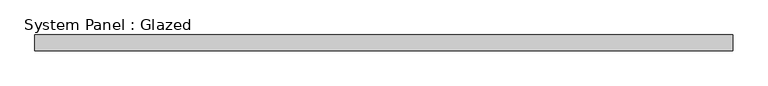
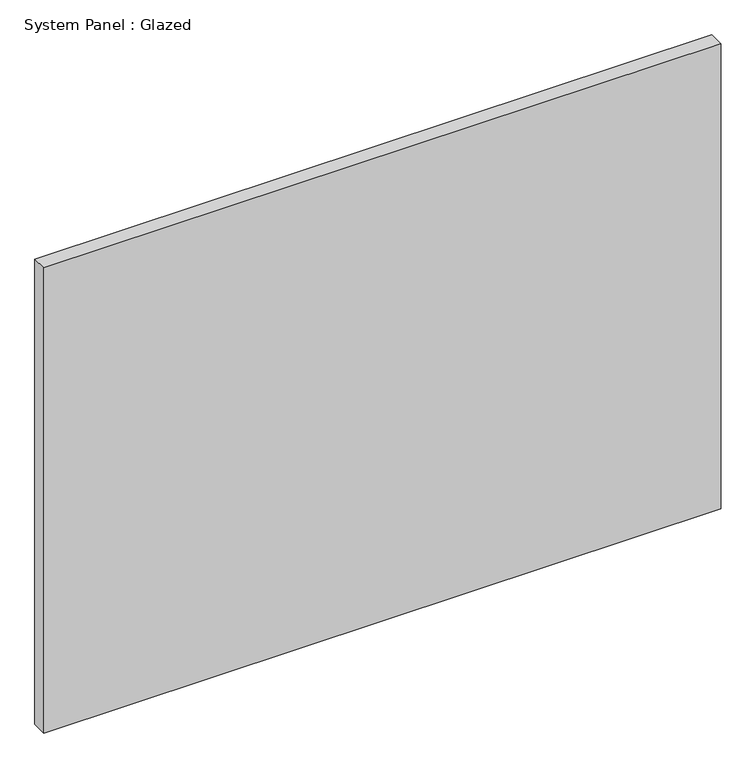
"""IFC4 building model written with IfcOpenShell, lengths in millimetres: plate geometry, System Panel : Glazed."""

from ifc_helpers import new_model, si_unit, origin, origin_with_axes, place, context, project, spatial, polyline, outline, extrude, source, transform, mapped, element, save


def system_panel_glazed_d044bda1(model_context):
    return source(origin(), model_context, "Body", "SweptSolid", [
        extrude(outline(polyline([(565.1499999, 19.05), (-565.1499999, 19.05), (-565.1499999, 44.45), (565.1499999, 44.45), (565.1499999, 19.05)])), origin_with_axes(), (0.0, 0.0, 1.0), 820.4497825),
    ])


if __name__ == "__main__":
    model = new_model("IFC4")
    model_context = context("Model", 3, world=origin())
    ifc_project = project(units=[si_unit("LENGTHUNIT", "METRE", prefix="MILLI")], contexts=[model_context])
    site = spatial("IfcSite", under=ifc_project)
    building = spatial("IfcBuilding", under=site)
    placement = place(None, origin())
    system_panel_glazed_shape = system_panel_glazed_d044bda1(model_context)
    element("IfcPlate", 1, ObjectType="System Panel : Glazed", at=placement, inside=building, context=model_context, shape_type="MappedRepresentation", body=[
        mapped(system_panel_glazed_shape, transform((0.0, 0.0, 0.0), x_axis=(1.0, 0.0, 0.0), y_axis=(0.0, 1.0, 0.0), z_axis=(0.0, 0.0, 1.0))),
    ])
    save(model, "model.ifc")

# Revit data of these elements
# Type "System Panel : Glazed"
#   Construction Type Id = "GSP4R"
#   Analytic Construction = "1/8 in Pilkington single glazing"
#   Visual Light Transmittance = 0.9
#   Solar Heat Gain Coefficient = 0.86
#   Heat Transfer Coefficient (U) = 1.18115 BTU/(h·ft²·°F)
#   Define Thermal Properties by = 1
# Element 1 (IfcPlate, "System Panel : Glazed")
#   Materials on its faces: "Glass"
# Materials
#   "Glass": class "Glass", colour RGB 0 128 192, transparency 0.75, Description = "Soda Lime Glass", Cost = 0
